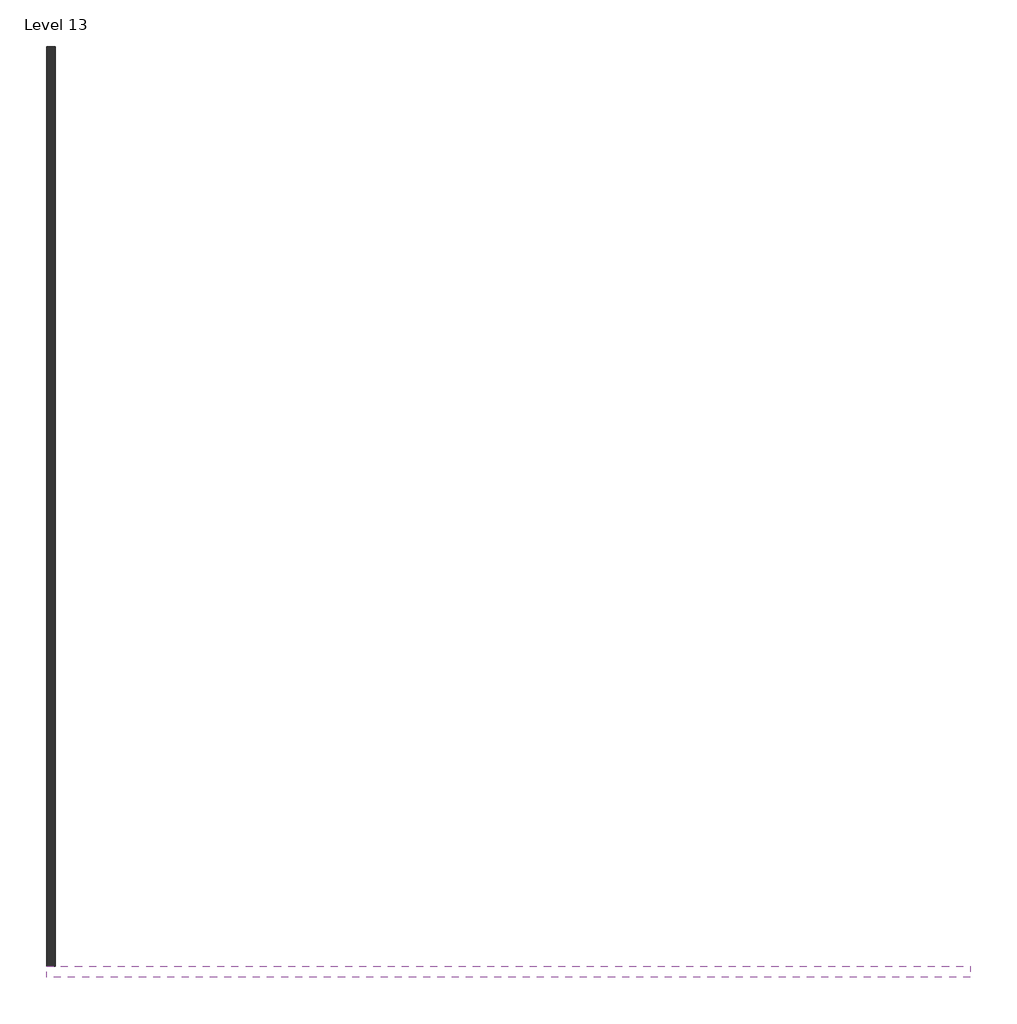
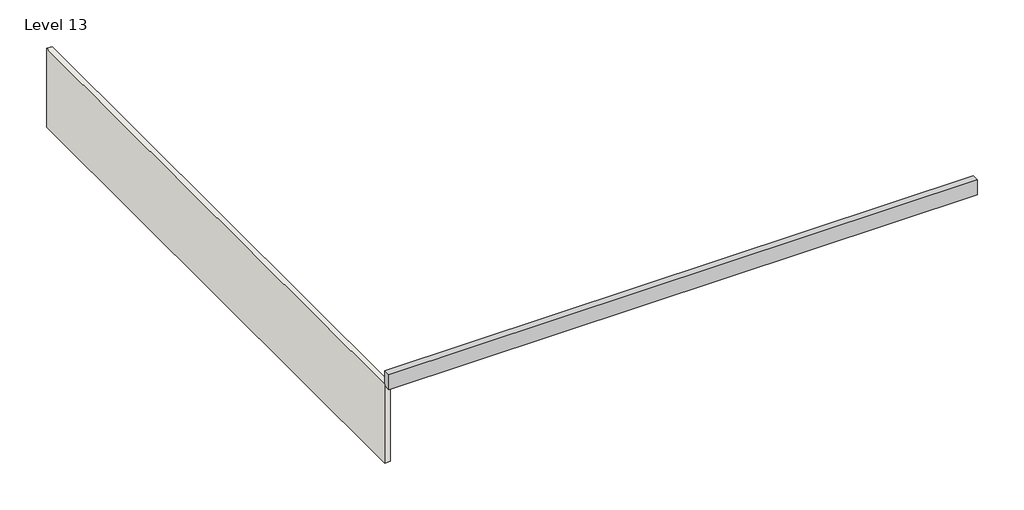
# One storey: 1 proxy, 1 wall.
"""IFC4 building model written with IfcOpenShell, lengths in millimetres."""

from ifc_helpers import new_model, si_unit, origin, place, context, project, spatial, faceted_brep, transform, mapped, element, save
from components import generic_models_9_generic_models_9_d1048e86

model = new_model("IFC4")

# Units and contexts
model_context = context("Model", 3, world=origin())
ifc_project = project(units=[si_unit("LENGTHUNIT", "METRE", prefix="MILLI")], contexts=[model_context])

# Site, building, storey
site = spatial("IfcSite", under=ifc_project)
building = spatial("IfcBuilding", under=site)
storey = spatial("IfcBuildingStorey", under=building, Name="Level 13", Elevation=19659.6)

# Proxy
placement = place(None, origin())
generic_models_9_generic_models_9_shape = generic_models_9_generic_models_9_d1048e86(model_context)
element("IfcBuildingElementProxy", 1, Name="Generic Models 9 : Generic Models 9", ObjectType="Generic Models 9 : Generic Models 9", at=placement, inside=storey, context=model_context, shape_type="MappedRepresentation", body=[
    mapped(generic_models_9_generic_models_9_shape, transform((0.0, 0.0, 0.0), x_axis=(1.0, 0.0, 0.0), y_axis=(0.0, 1.0, 0.0), z_axis=(0.0, 0.0, 1.0))),
])

# Wall
element("IfcWall", 2, ObjectType="outer wall", at=placement, inside=storey, context=model_context, shape_type="Brep", body=[
    faceted_brep([(-8731.5629849, -3682.5004242, 19659.6), (-8731.5629849, 17551.8995758, 19659.6), (-8731.5629849, 17755.0995758, 19659.6), (-8731.5629849, 17755.0995758, 22707.6), (-8731.5629849, 17551.8995758, 22707.6), (-8731.5629849, -3682.5004242, 22707.6), (-8934.7629849, -3682.5004242, 19659.6), (-8934.7629849, -3682.5004242, 22707.6), (-8934.7629849, 17551.8995758, 22707.6), (-8934.7629849, 17755.0995758, 22707.6), (-8934.7629849, 17755.0995758, 19659.6), (-8934.7629849, 17551.8995758, 19659.6)], [[[0, 1, 2, 3, 4, 5]], [[6, 7, 8, 9, 10, 11]], [[2, 1, 0, 6, 11, 10]], [[0, 5, 7, 6]], [[5, 4, 3, 9, 8, 7]], [[3, 2, 10, 9]]]),
])

save(model, "model.ifc")

# Revit data of these elements
# Type "outer wall"
#   Assembly Code = "B2010"
#   Layers, outside or top first: 0' - 8" "Copper" (function 1)
# Element 1 (IfcBuildingElementProxy, "Generic Models 9 : Generic Models 9")
#   Phase Created = New Construction
# Element 2 (IfcWall, "outer wall")
#   Top Offset = 0' - 0"
#   Base Offset = 0' - 0"
#   Unconnected Height = 10' - 0"
#   wall height = 10' - 0"
#   Phase Created = New Construction
#   Base Constraint = Level 13
#   Materials on its faces: "Copper"
# Materials
#   "Copper": class "Metal", colour RGB 0 0 0, transparency 0, Description = "Copper, matte finish", Cost = 0
